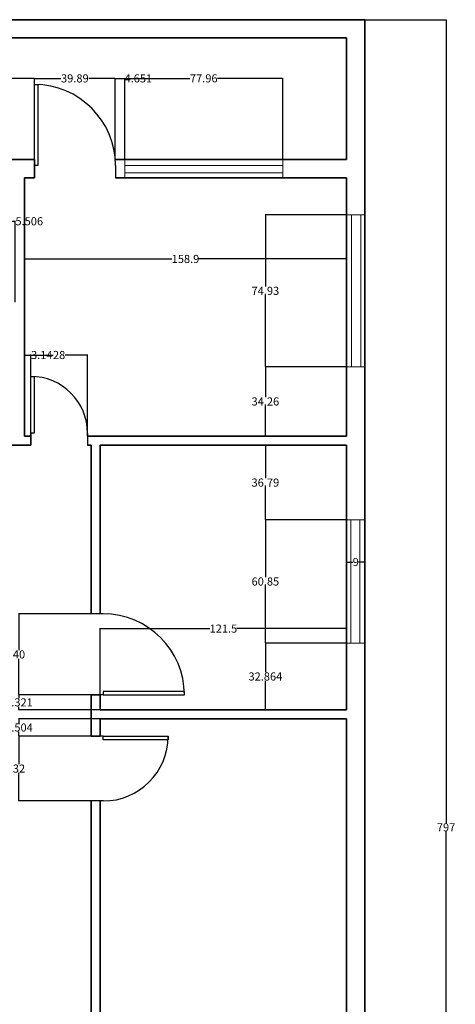
# Model space of a CAD drawing. Units: inches. Extents: x 1353 to 1853, y 16593 to 17433.
# Tile 4 of 4: x 1639 to 1853, y 16947 to 17433. Entities that reach past the tile are written whole.
import ezdxf

# ---------------------------------------------------------------- set-up
doc = ezdxf.new("R2010")
doc.units = ezdxf.units.IN
doc.header["$MEASUREMENT"] = 0
for name, color, linetype, lineweight in [('A-ANNO-DIMS', 2, 'Continuous', 18), ('A-DOOR', 3, 'Continuous', 25), ('A-GLAZ', 4, 'Continuous', 18), ('A-WALL', 7, 'Continuous', 35)]:
    doc.layers.add(name, color=color, linetype=linetype, lineweight=lineweight)
doc.styles.get("Standard").update_dxf_attribs({"font": 'arial.ttf'})
doc.dimstyles.get("Standard").update_dxf_attribs({"dimtxt": 4, "dimasz": 0.18, "dimexe": 0.18, "dimexo": 0.0625, "dimgap": 0.09, "dimtad": 0, "dimtih": 1, "dimtoh": 1, "dimdec": 0, "dimzin": 0, "dimdsep": 46, "dimlunit": 3, "dimtxsty": 'Standard', "dimcen": 0.09, "dimadec": 0, "dimazin": 0, "dimtfac": 1, "dimtdec": 0, "dimtofl": 0, "dimtmove": 0, "dimatfit": 3, "dimfxl": 1, "dimtolj": 1, "dimtzin": 0, "dimarcsym": 0})

# ---------------------------------------------------------------- blocks, each defined once
blk = doc.blocks.new('*U2')
for p, q in [((0, 0), (0, -6)), ((40, 0), (40, -6))]:
    blk.add_line(p, q)
blk.add_lwpolyline([(0, 0), (0, 40), (1.75, 40), (1.75, 0)], close=True)
blk.add_arc((0, 0), 40, 0, 90)
blk = doc.blocks.new('*U6')
for p, q in [((0, 0), (0, -6)), ((28, 0), (28, -6))]:
    blk.add_line(p, q)
blk.add_lwpolyline([(0, 0), (0, 28), (1.75, 28), (1.75, 0)], close=True)
blk.add_arc((0, 0), 28, 0, 90)
blk = doc.blocks.new('*U5')
for p, q in [((0, 0), (0, 6)), ((40, 0), (40, 6))]:
    blk.add_line(p, q)
blk.add_lwpolyline([(0, 0), (0, -40), (1.75, -40), (1.75, 0)], close=True)
blk.add_arc((0, 0), 40, 270, 0)
blk = doc.blocks.new('*U4')
for p, q in [((0, 0), (0, -6)), ((32, 0), (32, -6))]:
    blk.add_line(p, q)
blk.add_lwpolyline([(0, 0), (0, 32), (1.75, 32), (1.75, 0)], close=True)
blk.add_arc((0, 0), 32, 0, 90)
blk = doc.blocks.new('*D14')
at = {"layer": 'A-ANNO-DIMS', "color": 0, "lineweight": -2, "transparency": 16777216}
for p, q in [((1808.95, 17432.78), (1849.11, 17432.78)), ((1848.93, 17432.6), (1848.93, 17036.41)), ((1848.93, 16635.96), (1848.93, 17032.15)), ((1808.95, 16635.78), (1849.11, 16635.78))]:
    blk.add_line(p, q, dxfattribs=at)
at = {"layer": 'A-ANNO-DIMS', "color": 0, "transparency": 16777216}
for points in [[(1848.9, 17432.6), (1848.96, 17432.6), (1848.93, 17432.78)], [(1848.9, 16635.96), (1848.96, 16635.96), (1848.93, 16635.78)]]:
    blk.add_solid(points, dxfattribs=at)
at = {"layer": 'Defpoints', "color": 0, "transparency": 16777216}
for p in [(1808.88, 17432.78), (1848.93, 17432.78), (1808.88, 16635.78)]:
    blk.add_point(p, dxfattribs=at)
at = {"layer": 'A-ANNO-DIMS', "color": 0, "transparency": 16777216, "insert": (1848.93, 17034.28), "char_height": 4, "attachment_point": 5}
blk.add_mtext('\\A1;797', dxfattribs=at)
blk = doc.blocks.new('*D25')
at = {"layer": 'A-ANNO-DIMS', "color": 0, "lineweight": -2, "transparency": 16777216}
for p, q in [((1640.98, 17354.72), (1640.98, 17314.55)), ((1799.88, 17354.72), (1799.88, 17314.55)), ((1641.16, 17314.73), (1713.78, 17314.73)), ((1799.7, 17314.73), (1727.09, 17314.73))]:
    blk.add_line(p, q, dxfattribs=at)
at = {"layer": 'A-ANNO-DIMS', "color": 0, "transparency": 16777216}
for points in [[(1641.16, 17314.76), (1641.16, 17314.7), (1640.98, 17314.73)], [(1799.7, 17314.76), (1799.7, 17314.7), (1799.88, 17314.73)]]:
    blk.add_solid(points, dxfattribs=at)
at = {"layer": 'Defpoints', "color": 0, "transparency": 16777216}
for p in [(1640.98, 17354.78), (1799.88, 17354.78), (1640.98, 17314.73)]:
    blk.add_point(p, dxfattribs=at)
at = {"layer": 'A-ANNO-DIMS', "color": 0, "transparency": 16777216, "insert": (1720.43, 17314.73), "char_height": 4, "attachment_point": 5}
blk.add_mtext('\\A1;158.9', dxfattribs=at)
blk = doc.blocks.new('*D28')
at = {"layer": 'A-ANNO-DIMS', "color": 0, "lineweight": -2, "transparency": 16777216}
for p, q in [((1678.38, 17092.34), (1678.38, 17132.51)), ((1678.56, 17132.33), (1732.47, 17132.33)), ((1799.7, 17132.33), (1745.8, 17132.33)), ((1799.88, 17092.34), (1799.88, 17132.51))]:
    blk.add_line(p, q, dxfattribs=at)
at = {"layer": 'A-ANNO-DIMS', "color": 0, "transparency": 16777216}
for points in [[(1678.56, 17132.36), (1678.56, 17132.3), (1678.38, 17132.33)], [(1799.7, 17132.36), (1799.7, 17132.3), (1799.88, 17132.33)]]:
    blk.add_solid(points, dxfattribs=at)
at = {"layer": 'Defpoints', "color": 0, "transparency": 16777216}
for p in [(1799.88, 17132.33), (1678.38, 17092.28), (1799.88, 17092.28)]:
    blk.add_point(p, dxfattribs=at)
at = {"layer": 'A-ANNO-DIMS', "color": 0, "transparency": 16777216, "insert": (1739.13, 17132.33), "char_height": 4, "attachment_point": 5}
blk.add_mtext('\\A1;121.5', dxfattribs=at)
blk = doc.blocks.new('*D35')
at = {"layer": 'A-ANNO-DIMS', "color": 0, "lineweight": -2, "transparency": 16777216}
for p, q in [((1645.93, 17363.84), (1645.93, 17404.01)), ((1646.11, 17403.83), (1659.03, 17403.83)), ((1685.64, 17403.83), (1672.72, 17403.83)), ((1685.82, 17363.84), (1685.82, 17404.01))]:
    blk.add_line(p, q, dxfattribs=at)
at = {"layer": 'A-ANNO-DIMS', "color": 0, "transparency": 16777216}
for points in [[(1646.11, 17403.86), (1646.11, 17403.8), (1645.93, 17403.83)], [(1685.64, 17403.86), (1685.64, 17403.8), (1685.82, 17403.83)]]:
    blk.add_solid(points, dxfattribs=at)
at = {"layer": 'Defpoints', "color": 0, "transparency": 16777216}
for p in [(1685.82, 17403.83), (1645.93, 17363.78), (1685.82, 17363.78)]:
    blk.add_point(p, dxfattribs=at)
at = {"layer": 'A-ANNO-DIMS', "color": 0, "transparency": 16777216, "insert": (1665.87, 17403.83), "char_height": 4, "attachment_point": 5}
blk.add_mtext('\\A1;39.89', dxfattribs=at)
blk = doc.blocks.new('*D36')
at = {"layer": 'A-ANNO-DIMS', "color": 0, "lineweight": -2, "transparency": 16777216}
for p, q in [((1690.47, 17363.84), (1690.47, 17404.01)), ((1690.65, 17403.83), (1722.63, 17403.83)), ((1768.25, 17403.83), (1736.27, 17403.83)), ((1768.43, 17363.84), (1768.43, 17404.01))]:
    blk.add_line(p, q, dxfattribs=at)
at = {"layer": 'A-ANNO-DIMS', "color": 0, "transparency": 16777216}
for points in [[(1690.65, 17403.86), (1690.65, 17403.8), (1690.47, 17403.83)], [(1768.25, 17403.86), (1768.25, 17403.8), (1768.43, 17403.83)]]:
    blk.add_solid(points, dxfattribs=at)
at = {"layer": 'Defpoints', "color": 0, "transparency": 16777216}
for p in [(1768.43, 17403.83), (1690.47, 17363.78), (1768.43, 17363.78)]:
    blk.add_point(p, dxfattribs=at)
at = {"layer": 'A-ANNO-DIMS', "color": 0, "transparency": 16777216, "insert": (1729.45, 17403.83), "char_height": 4, "attachment_point": 5}
blk.add_mtext('\\A1;77.96', dxfattribs=at)
blk = doc.blocks.new('*D40')
at = {"layer": 'A-ANNO-DIMS', "color": 0, "lineweight": -2, "transparency": 16777216}
for p, q in [((1604.95, 17363.84), (1604.95, 17404.01)), ((1605.13, 17403.83), (1618.52, 17403.83)), ((1645.75, 17403.83), (1632.36, 17403.83)), ((1645.93, 17363.84), (1645.93, 17404.01))]:
    blk.add_line(p, q, dxfattribs=at)
at = {"layer": 'A-ANNO-DIMS', "color": 0, "transparency": 16777216}
for points in [[(1605.13, 17403.86), (1605.13, 17403.8), (1604.95, 17403.83)], [(1645.75, 17403.86), (1645.75, 17403.8), (1645.93, 17403.83)]]:
    blk.add_solid(points, dxfattribs=at)
at = {"layer": 'Defpoints', "color": 0, "transparency": 16777216}
for p in [(1645.93, 17403.83), (1604.95, 17363.78), (1645.93, 17363.78)]:
    blk.add_point(p, dxfattribs=at)
at = {"layer": 'A-ANNO-DIMS', "color": 0, "transparency": 16777216, "insert": (1625.44, 17403.83), "char_height": 4, "attachment_point": 5}
blk.add_mtext('\\A1;40.98', dxfattribs=at)
blk = doc.blocks.new('*D41')
at = {"layer": 'A-ANNO-DIMS', "color": 0, "lineweight": -2, "transparency": 16777216}
for p, q in [((1685.82, 17363.84), (1685.82, 17404.01)), ((1686, 17403.83), (1690.29, 17403.83)), ((1690.47, 17363.84), (1690.47, 17404.01)), ((1690.47, 17403.83), (1690.65, 17403.83))]:
    blk.add_line(p, q, dxfattribs=at)
at = {"layer": 'A-ANNO-DIMS', "color": 0, "transparency": 16777216}
for points in [[(1686, 17403.86), (1686, 17403.8), (1685.82, 17403.83)], [(1690.29, 17403.86), (1690.29, 17403.8), (1690.47, 17403.83)]]:
    blk.add_solid(points, dxfattribs=at)
at = {"layer": 'Defpoints', "color": 0, "transparency": 16777216}
for p in [(1690.47, 17403.83), (1685.82, 17363.78), (1690.47, 17363.78)]:
    blk.add_point(p, dxfattribs=at)
at = {"layer": 'A-ANNO-DIMS', "color": 0, "transparency": 16777216, "insert": (1697.18, 17403.83), "char_height": 4, "attachment_point": 5}
blk.add_mtext('\\A1;4.651', dxfattribs=at)
blk = doc.blocks.new('*D42')
at = {"layer": 'A-ANNO-DIMS', "color": 0, "lineweight": -2, "transparency": 16777216}
for p, q in [((1799.82, 17336.46), (1759.65, 17336.46)), ((1759.83, 17336.28), (1759.83, 17301.13)), ((1759.83, 17261.72), (1759.83, 17296.87)), ((1799.82, 17261.54), (1759.65, 17261.54))]:
    blk.add_line(p, q, dxfattribs=at)
at = {"layer": 'A-ANNO-DIMS', "color": 0, "transparency": 16777216}
for points in [[(1759.8, 17336.28), (1759.86, 17336.28), (1759.83, 17336.46)], [(1759.8, 17261.72), (1759.86, 17261.72), (1759.83, 17261.54)]]:
    blk.add_solid(points, dxfattribs=at)
at = {"layer": 'Defpoints', "color": 0, "transparency": 16777216}
for p in [(1759.83, 17336.46), (1799.88, 17336.46), (1799.88, 17261.54)]:
    blk.add_point(p, dxfattribs=at)
at = {"layer": 'A-ANNO-DIMS', "color": 0, "transparency": 16777216, "insert": (1759.83, 17299), "char_height": 4, "attachment_point": 5}
blk.add_mtext('\\A1;74.93', dxfattribs=at)
blk = doc.blocks.new('*D43')
at = {"layer": 'A-ANNO-DIMS', "color": 0, "lineweight": -2, "transparency": 16777216}
for p, q in [((1799.82, 17261.54), (1759.65, 17261.54)), ((1759.83, 17261.36), (1759.83, 17246.54)), ((1759.83, 17227.46), (1759.83, 17242.28)), ((1799.82, 17227.28), (1759.65, 17227.28))]:
    blk.add_line(p, q, dxfattribs=at)
at = {"layer": 'A-ANNO-DIMS', "color": 0, "transparency": 16777216}
for points in [[(1759.8, 17261.36), (1759.86, 17261.36), (1759.83, 17261.54)], [(1759.8, 17227.46), (1759.86, 17227.46), (1759.83, 17227.28)]]:
    blk.add_solid(points, dxfattribs=at)
at = {"layer": 'Defpoints', "color": 0, "transparency": 16777216}
for p in [(1759.83, 17261.54), (1799.88, 17261.54), (1799.88, 17227.28)]:
    blk.add_point(p, dxfattribs=at)
at = {"layer": 'A-ANNO-DIMS', "color": 0, "transparency": 16777216, "insert": (1759.83, 17244.41), "char_height": 4, "attachment_point": 5}
blk.add_mtext('\\A1;34.26', dxfattribs=at)
blk = doc.blocks.new('*D44')
at = {"layer": 'A-ANNO-DIMS', "color": 0, "lineweight": -2, "transparency": 16777216}
for p, q in [((1799.82, 17185.99), (1759.65, 17185.99)), ((1759.83, 17185.81), (1759.83, 17157.7)), ((1759.83, 17125.32), (1759.83, 17153.44)), ((1799.82, 17125.14), (1759.65, 17125.14))]:
    blk.add_line(p, q, dxfattribs=at)
at = {"layer": 'A-ANNO-DIMS', "color": 0, "transparency": 16777216}
for points in [[(1759.8, 17185.81), (1759.86, 17185.81), (1759.83, 17185.99)], [(1759.8, 17125.32), (1759.86, 17125.32), (1759.83, 17125.14)]]:
    blk.add_solid(points, dxfattribs=at)
at = {"layer": 'Defpoints', "color": 0, "transparency": 16777216}
for p in [(1759.83, 17185.99), (1799.88, 17185.99), (1799.88, 17125.14)]:
    blk.add_point(p, dxfattribs=at)
at = {"layer": 'A-ANNO-DIMS', "color": 0, "transparency": 16777216, "insert": (1759.83, 17155.57), "char_height": 4, "attachment_point": 5}
blk.add_mtext('\\A1;60.85', dxfattribs=at)
blk = doc.blocks.new('*D45')
at = {"layer": 'A-ANNO-DIMS', "color": 0, "lineweight": -2, "transparency": 16777216}
for p, q in [((1799.82, 17125.14), (1759.65, 17125.14)), ((1759.83, 17124.96), (1759.83, 17110.85)), ((1759.83, 17092.46), (1759.83, 17106.58)), ((1799.82, 17092.28), (1759.65, 17092.28))]:
    blk.add_line(p, q, dxfattribs=at)
at = {"layer": 'A-ANNO-DIMS', "color": 0, "transparency": 16777216}
for points in [[(1759.8, 17124.96), (1759.86, 17124.96), (1759.83, 17125.14)], [(1759.8, 17092.46), (1759.86, 17092.46), (1759.83, 17092.28)]]:
    blk.add_solid(points, dxfattribs=at)
at = {"layer": 'Defpoints', "color": 0, "transparency": 16777216}
for p in [(1759.83, 17125.14), (1799.88, 17125.14), (1799.88, 17092.28)]:
    blk.add_point(p, dxfattribs=at)
at = {"layer": 'A-ANNO-DIMS', "color": 0, "transparency": 16777216, "insert": (1759.83, 17108.71), "char_height": 4, "attachment_point": 5}
blk.add_mtext('\\A1;32.864', dxfattribs=at)
blk = doc.blocks.new('*D46')
at = {"layer": 'A-ANNO-DIMS', "color": 0, "lineweight": -2, "transparency": 16777216}
for p, q in [((1799.82, 17222.78), (1759.65, 17222.78)), ((1759.83, 17222.6), (1759.83, 17206.52)), ((1759.83, 17186.17), (1759.83, 17202.25)), ((1799.82, 17185.99), (1759.65, 17185.99))]:
    blk.add_line(p, q, dxfattribs=at)
at = {"layer": 'A-ANNO-DIMS', "color": 0, "transparency": 16777216}
for points in [[(1759.8, 17222.6), (1759.86, 17222.6), (1759.83, 17222.78)], [(1759.8, 17186.17), (1759.86, 17186.17), (1759.83, 17185.99)]]:
    blk.add_solid(points, dxfattribs=at)
at = {"layer": 'Defpoints', "color": 0, "transparency": 16777216}
for p in [(1759.83, 17222.78), (1799.88, 17222.78), (1799.88, 17185.99)]:
    blk.add_point(p, dxfattribs=at)
at = {"layer": 'A-ANNO-DIMS', "color": 0, "transparency": 16777216, "insert": (1759.83, 17204.39), "char_height": 4, "attachment_point": 5}
blk.add_mtext('\\A1;36.79', dxfattribs=at)
blk = doc.blocks.new('*D52')
at = {"layer": 'A-ANNO-DIMS', "color": 0, "lineweight": -2, "transparency": 16777216}
for p, q in [((1630.88, 17293.34), (1630.88, 17333.51)), ((1631.06, 17333.33), (1636.2, 17333.33)), ((1636.38, 17293.34), (1636.38, 17333.51)), ((1636.38, 17333.33), (1636.56, 17333.33))]:
    blk.add_line(p, q, dxfattribs=at)
at = {"layer": 'A-ANNO-DIMS', "color": 0, "transparency": 16777216}
for points in [[(1631.06, 17333.36), (1631.06, 17333.3), (1630.88, 17333.33)], [(1636.2, 17333.36), (1636.2, 17333.3), (1636.38, 17333.33)]]:
    blk.add_solid(points, dxfattribs=at)
at = {"layer": 'Defpoints', "color": 0, "transparency": 16777216}
for p in [(1636.38, 17333.33), (1630.88, 17293.28), (1636.38, 17293.28)]:
    blk.add_point(p, dxfattribs=at)
at = {"layer": 'A-ANNO-DIMS', "color": 0, "transparency": 16777216, "insert": (1643.4, 17333.33), "char_height": 4, "attachment_point": 5}
blk.add_mtext('\\A1;5.506', dxfattribs=at)
blk = doc.blocks.new('*D53')
at = {"layer": 'A-ANNO-DIMS', "color": 0, "lineweight": -2, "transparency": 16777216}
for p, q in [((1644.12, 17227.34), (1644.12, 17267.51)), ((1644.3, 17267.33), (1655.13, 17267.33)), ((1671.94, 17267.33), (1661.12, 17267.33)), ((1672.12, 17227.34), (1672.12, 17267.51))]:
    blk.add_line(p, q, dxfattribs=at)
at = {"layer": 'A-ANNO-DIMS', "color": 0, "transparency": 16777216}
for points in [[(1644.3, 17267.36), (1644.3, 17267.3), (1644.12, 17267.33)], [(1671.94, 17267.36), (1671.94, 17267.3), (1672.12, 17267.33)]]:
    blk.add_solid(points, dxfattribs=at)
at = {"layer": 'Defpoints', "color": 0, "transparency": 16777216}
for p in [(1672.12, 17267.33), (1644.12, 17227.28), (1672.12, 17227.28)]:
    blk.add_point(p, dxfattribs=at)
at = {"layer": 'A-ANNO-DIMS', "color": 0, "transparency": 16777216, "insert": (1658.12, 17267.33), "char_height": 4, "attachment_point": 5}
blk.add_mtext('\\A1;28', dxfattribs=at)
blk = doc.blocks.new('*D54')
at = {"layer": 'A-ANNO-DIMS', "color": 0, "lineweight": -2, "transparency": 16777216}
for p, q in [((1640.98, 17227.34), (1640.98, 17267.51)), ((1641.16, 17267.33), (1643.94, 17267.33)), ((1644.12, 17227.34), (1644.12, 17267.51)), ((1644.12, 17267.33), (1644.3, 17267.33))]:
    blk.add_line(p, q, dxfattribs=at)
at = {"layer": 'A-ANNO-DIMS', "color": 0, "transparency": 16777216}
for points in [[(1641.16, 17267.36), (1641.16, 17267.3), (1640.98, 17267.33)], [(1643.94, 17267.36), (1643.94, 17267.3), (1644.12, 17267.33)]]:
    blk.add_solid(points, dxfattribs=at)
at = {"layer": 'Defpoints', "color": 0, "transparency": 16777216}
for p in [(1644.12, 17267.33), (1640.98, 17227.28), (1644.12, 17227.28)]:
    blk.add_point(p, dxfattribs=at)
at = {"layer": 'A-ANNO-DIMS', "color": 0, "transparency": 16777216, "insert": (1649.58, 17267.33), "char_height": 4, "attachment_point": 5}
blk.add_mtext('\\A1;3.14', dxfattribs=at)
blk = doc.blocks.new('*D61')
at = {"layer": 'A-ANNO-DIMS', "color": 0, "lineweight": -2, "transparency": 16777216}
for p, q in [((1678.32, 17139.6), (1638.15, 17139.6)), ((1638.33, 17139.42), (1638.33, 17121.73)), ((1638.33, 17099.78), (1638.33, 17117.47)), ((1678.32, 17099.6), (1638.15, 17099.6))]:
    blk.add_line(p, q, dxfattribs=at)
at = {"layer": 'A-ANNO-DIMS', "color": 0, "transparency": 16777216}
for points in [[(1638.3, 17139.42), (1638.36, 17139.42), (1638.33, 17139.6)], [(1638.3, 17099.78), (1638.36, 17099.78), (1638.33, 17099.6)]]:
    blk.add_solid(points, dxfattribs=at)
at = {"layer": 'Defpoints', "color": 0, "transparency": 16777216}
for p in [(1638.33, 17139.6), (1678.38, 17139.6), (1678.38, 17099.6)]:
    blk.add_point(p, dxfattribs=at)
at = {"layer": 'A-ANNO-DIMS', "color": 0, "transparency": 16777216, "insert": (1638.33, 17119.6), "char_height": 4, "attachment_point": 5}
blk.add_mtext('\\A1;40', dxfattribs=at)
blk = doc.blocks.new('*D62')
at = {"layer": 'A-ANNO-DIMS', "color": 0, "lineweight": -2, "transparency": 16777216}
for p, q in [((1678.32, 17079.28), (1638.15, 17079.28)), ((1638.33, 17079.1), (1638.33, 17065.41)), ((1638.33, 17047.46), (1638.33, 17061.14)), ((1678.32, 17047.28), (1638.15, 17047.28))]:
    blk.add_line(p, q, dxfattribs=at)
at = {"layer": 'A-ANNO-DIMS', "color": 0, "transparency": 16777216}
for points in [[(1638.3, 17079.1), (1638.36, 17079.1), (1638.33, 17079.28)], [(1638.3, 17047.46), (1638.36, 17047.46), (1638.33, 17047.28)]]:
    blk.add_solid(points, dxfattribs=at)
at = {"layer": 'Defpoints', "color": 0, "transparency": 16777216}
for p in [(1638.33, 17079.28), (1678.38, 17079.28), (1678.38, 17047.28)]:
    blk.add_point(p, dxfattribs=at)
at = {"layer": 'A-ANNO-DIMS', "color": 0, "transparency": 16777216, "insert": (1638.33, 17063.28), "char_height": 4, "attachment_point": 5}
blk.add_mtext('\\A1;32', dxfattribs=at)
blk = doc.blocks.new('*D74')
at = {"layer": 'A-ANNO-DIMS', "color": 0, "lineweight": -2, "transparency": 16777216}
for p, q in [((1678.32, 17087.78), (1638.15, 17087.78)), ((1638.33, 17087.6), (1638.33, 17085.66)), ((1678.32, 17079.28), (1638.15, 17079.28)), ((1638.33, 17079.46), (1638.33, 17081.4))]:
    blk.add_line(p, q, dxfattribs=at)
at = {"layer": 'A-ANNO-DIMS', "color": 0, "transparency": 16777216}
for points in [[(1638.3, 17087.6), (1638.36, 17087.6), (1638.33, 17087.78)], [(1638.3, 17079.46), (1638.36, 17079.46), (1638.33, 17079.28)]]:
    blk.add_solid(points, dxfattribs=at)
at = {"layer": 'Defpoints', "color": 0, "transparency": 16777216}
for p in [(1638.33, 17087.78), (1678.38, 17087.78), (1678.38, 17079.28)]:
    blk.add_point(p, dxfattribs=at)
at = {"layer": 'A-ANNO-DIMS', "color": 0, "transparency": 16777216, "insert": (1638.33, 17083.53), "char_height": 4, "attachment_point": 5}
blk.add_mtext('\\A1;8.504', dxfattribs=at)
blk = doc.blocks.new('*D75')
at = {"layer": 'A-ANNO-DIMS', "color": 0, "lineweight": -2, "transparency": 16777216}
for p, q in [((1678.32, 17099.6), (1638.15, 17099.6)), ((1638.33, 17099.42), (1638.33, 17098.08)), ((1678.32, 17092.28), (1638.15, 17092.28)), ((1638.33, 17092.46), (1638.33, 17093.81))]:
    blk.add_line(p, q, dxfattribs=at)
at = {"layer": 'A-ANNO-DIMS', "color": 0, "transparency": 16777216}
for points in [[(1638.3, 17099.42), (1638.36, 17099.42), (1638.33, 17099.6)], [(1638.3, 17092.46), (1638.36, 17092.46), (1638.33, 17092.28)]]:
    blk.add_solid(points, dxfattribs=at)
at = {"layer": 'Defpoints', "color": 0, "transparency": 16777216}
for p in [(1638.33, 17099.6), (1678.38, 17099.6), (1678.38, 17092.28)]:
    blk.add_point(p, dxfattribs=at)
at = {"layer": 'A-ANNO-DIMS', "color": 0, "transparency": 16777216, "insert": (1638.33, 17095.94), "char_height": 4, "attachment_point": 5}
blk.add_mtext('\\A1;7.321', dxfattribs=at)
blk = doc.blocks.new('*D78')
at = {"layer": 'A-ANNO-DIMS', "color": 0, "lineweight": -2, "transparency": 16777216}
for p, q in [((1799.88, 17125.21), (1799.88, 17165.37)), ((1800.06, 17165.19), (1802.98, 17165.19)), ((1808.7, 17165.19), (1805.79, 17165.19)), ((1808.88, 17125.21), (1808.88, 17165.37))]:
    blk.add_line(p, q, dxfattribs=at)
at = {"layer": 'A-ANNO-DIMS', "color": 0, "transparency": 16777216}
for points in [[(1800.06, 17165.22), (1800.06, 17165.16), (1799.88, 17165.19)], [(1808.7, 17165.22), (1808.7, 17165.16), (1808.88, 17165.19)]]:
    blk.add_solid(points, dxfattribs=at)
at = {"layer": 'Defpoints', "color": 0, "transparency": 16777216}
for p in [(1808.88, 17165.19), (1799.88, 17125.14), (1808.88, 17125.14)]:
    blk.add_point(p, dxfattribs=at)
at = {"layer": 'A-ANNO-DIMS', "color": 0, "transparency": 16777216, "insert": (1804.38, 17165.19), "char_height": 4, "attachment_point": 5}
blk.add_mtext('\\A1;9', dxfattribs=at)

msp = doc.modelspace()

# ---------------------------------------------------------------- linework, layer by layer
at = {"layer": 'A-GLAZ'}
for p, q in [((1690.4681, 17363.7809), (1690.4681, 17354.7809)), ((1768.4275, 17363.7809), (1690.4681, 17363.7809)), ((1690.4681, 17363.7809), (1690.4681, 17360.9071)), ((1768.4275, 17354.7809), (1768.4275, 17363.7809)), ((1690.4681, 17360.9071), (1768.4275, 17360.9071)), ((1768.4275, 17360.9071), (1768.4275, 17357.2518)), ((1768.4275, 17357.2518), (1690.4681, 17357.2518)), ((1690.4681, 17354.7809), (1768.4275, 17354.7809)), ((1799.8844, 17336.4635), (1808.8844, 17336.4635)), ((1799.8844, 17261.5382), (1799.8844, 17336.4635)), ((1799.8844, 17336.4635), (1802.3172, 17336.4635)), ((1802.3172, 17336.4635), (1802.3172, 17261.5382)), ((1806.8587, 17261.5382), (1806.8587, 17336.4635)), ((1808.8844, 17336.4635), (1808.8844, 17261.5382)), ((1808.8844, 17261.5382), (1799.8844, 17261.5382)), ((1802.3172, 17261.5382), (1806.8587, 17261.5382)), ((1799.8844, 17185.9944), (1808.8844, 17185.9944)), ((1799.8844, 17125.1449), (1799.8844, 17185.9944)), ((1799.8844, 17185.9944), (1801.8923, 17185.9944)), ((1801.8923, 17185.9944), (1801.8923, 17125.1449)), ((1806.3721, 17125.1449), (1806.3721, 17185.9944)), ((1808.8844, 17185.9944), (1808.8844, 17125.1449)), ((1808.8844, 17125.1449), (1799.8844, 17125.1449)), ((1801.8923, 17125.1449), (1806.3721, 17125.1449))]:
    msp.add_line(p, q, dxfattribs=at)
at = {"layer": 'A-WALL'}
for p, q in [((1388.8844, 17432.7809), (1808.8844, 17432.7809)), ((1808.8844, 17432.7809), (1808.8844, 16635.7809)), ((1397.8844, 17423.7809), (1799.8844, 17423.7809)), ((1799.8844, 17423.7809), (1799.8844, 17363.7809)), ((1459.183, 17363.7809), (1645.9302, 17363.7809)), ((1645.9302, 17354.7809), (1645.9302, 17363.7809)), ((1688.5176, 17363.7809), (1685.8175, 17363.7809)), ((1688.5176, 17363.7809), (1799.8844, 17363.7809)), ((1640.9844, 17227.2809), (1640.9844, 17354.7809)), ((1640.9844, 17354.7809), (1645.9302, 17354.7809)), ((1690.4681, 17354.7809), (1685.9302, 17354.7809)), ((1688.5176, 17354.7809), (1799.8844, 17354.7809)), ((1799.8844, 17354.7809), (1799.8844, 17227.2809)), ((1640.9844, 17227.2809), (1644.1249, 17227.2809)), ((1644.1249, 17222.7809), (1644.1249, 17227.2809)), ((1672.1249, 17227.2809), (1799.8844, 17227.2809)), ((1528.3844, 17222.7809), (1640.9844, 17222.7809)), ((1640.9844, 17222.7809), (1644.1249, 17222.7809)), ((1672.1249, 17222.7809), (1673.8844, 17222.7809)), ((1673.8844, 17222.7809), (1673.8844, 17139.6023)), ((1678.3844, 17222.7809), (1678.3844, 17139.6023)), ((1678.3844, 17222.7809), (1799.8844, 17222.7809)), ((1799.8844, 17222.7809), (1799.8844, 17092.2809)), ((1678.3844, 17099.6023), (1673.8844, 17099.6023)), ((1673.8844, 17087.7809), (1673.8844, 17099.6023)), ((1673.8844, 17099.6023), (1678.3844, 17099.6023)), ((1678.3844, 17099.6023), (1678.3844, 17092.2809)), ((1678.3844, 17092.2809), (1799.8844, 17092.2809)), ((1673.8844, 17087.7809), (1673.8844, 17079.277)), ((1678.3844, 17087.7809), (1799.8844, 17087.7809)), ((1678.3844, 17087.7809), (1678.3844, 17079.277)), ((1799.8844, 17087.7809), (1799.8844, 16644.7809)), ((1678.3844, 17079.277), (1673.8844, 17079.277)), ((1673.8844, 16893.7809), (1673.8844, 17047.277)), ((1678.3844, 16759.1207), (1678.3844, 17047.277))]:
    msp.add_line(p, q, dxfattribs=at)

# ---------------------------------------------------------------- block references
at = {"layer": 'A-DOOR'}
for name, p in [('*U2', (1645.9302, 17360.7809)), ('*U6', (1644.1249, 17228.7809))]:
    msp.add_blockref(name, p, dxfattribs=at)
for name, p, rotation in [('*U5', (1679.8844, 17099.6023), 90), ('*U4', (1679.8844, 17079.277), 270.0000000000025)]:
    msp.add_blockref(name, p, dxfattribs=dict(at, rotation=rotation))

# ---------------------------------------------------------------- dimensions: what is measured, and where the dimension line sits
at = {"layer": 'A-ANNO-DIMS'}
for base, p1, p2, angle, override, picture, middle in [((1848.9344, 17432.7809), (1808.8844, 16635.7809), (1808.8844, 17432.7809), 90, {"dimdec": 0, "dimlfac": 1, "dimrnd": 0, "dimzin": 0, "dimdsep": 46, "dimlunit": 2}, '*D14', (1848.9344, 17034.2809)), ((1640.9844, 17314.7309), (1799.8844, 17354.7809), (1640.9844, 17354.7809), 180, {"dimdec": 1, "dimlfac": 1, "dimrnd": 0, "dimzin": 0, "dimdsep": 46, "dimlunit": 2}, '*D25', (1720.4344, 17314.7309)), ((1759.8344, 17336.4635), (1799.8844, 17261.5382), (1799.8844, 17336.4635), 90, {"dimdec": 2, "dimlfac": 1, "dimrnd": 0, "dimzin": 0, "dimdsep": 46, "dimlunit": 2}, '*D42', (1759.8344, 17299.0008)), ((1759.8344, 17261.5382), (1799.8844, 17227.2809), (1799.8844, 17261.5382), 90, {"dimdec": 2, "dimlfac": 1, "dimrnd": 0, "dimzin": 0, "dimdsep": 46, "dimlunit": 2}, '*D43', (1759.8344, 17244.4096)), ((1759.8344, 17222.7809), (1799.8844, 17185.9944), (1799.8844, 17222.7809), 90, {"dimdec": 2, "dimlfac": 1, "dimrnd": 0, "dimzin": 0, "dimdsep": 46, "dimlunit": 2}, '*D46', (1759.8344, 17204.3877)), ((1759.8344, 17185.9944), (1799.8844, 17125.1449), (1799.8844, 17185.9944), 90, {"dimdec": 2, "dimlfac": 1, "dimrnd": 0, "dimzin": 0, "dimdsep": 46, "dimlunit": 2}, '*D44', (1759.8344, 17155.5696)), ((1638.3344, 17139.6023), (1678.3844, 17099.6023), (1678.3844, 17139.6023), 90, {"dimdec": 0, "dimlfac": 1, "dimrnd": 0, "dimzin": 0, "dimdsep": 46, "dimlunit": 2}, '*D61', (1638.3344, 17119.6023)), ((1759.8344, 17125.1449), (1799.8844, 17092.2809), (1799.8844, 17125.1449), 90, {"dimdec": 3, "dimlfac": 1, "dimrnd": 0, "dimzin": 0, "dimdsep": 46, "dimlunit": 2}, '*D45', (1759.8344, 17108.7129)), ((1638.3344, 17099.6023), (1678.3844, 17092.2809), (1678.3844, 17099.6023), 90, {"dimdec": 3, "dimlfac": 1, "dimrnd": 0, "dimzin": 0, "dimdsep": 46, "dimlunit": 2}, '*D75', (1638.3344, 17095.9416)), ((1638.3344, 17087.7809), (1678.3844, 17079.277), (1678.3844, 17087.7809), 90, {"dimdec": 3, "dimlfac": 1, "dimrnd": 0, "dimzin": 0, "dimdsep": 46, "dimlunit": 2}, '*D74', (1638.3344, 17083.529)), ((1638.3344, 17079.277), (1678.3844, 17047.277), (1678.3844, 17079.277), 90, {"dimdec": 0, "dimlfac": 1, "dimrnd": 0, "dimzin": 0, "dimdsep": 46, "dimlunit": 2}, '*D62', (1638.3344, 17063.277))]:
    dim = msp.add_linear_dim(base=base, p1=p1, p2=p2, angle=angle, dimstyle='Standard', override=override, dxfattribs=at)
    dim.commit()
    dim.dimension.update_dxf_attribs({"geometry": picture, "text_midpoint": middle})
for base, p1, p2, override, picture, middle in [((1645.9302, 17403.8309), (1604.9522, 17363.7809), (1645.9302, 17363.7809), {"dimdec": 2, "dimlfac": 1, "dimrnd": 0, "dimzin": 0, "dimdsep": 46, "dimlunit": 2}, '*D40', (1625.4412, 17403.8309)), ((1685.8175, 17403.8309), (1645.9302, 17363.7809), (1685.8175, 17363.7809), {"dimdec": 2, "dimlfac": 1, "dimrnd": 0, "dimzin": 0, "dimdsep": 46, "dimlunit": 2}, '*D35', (1665.8739, 17403.8309)), ((1690.4681, 17403.8309), (1685.8175, 17363.7809), (1690.4681, 17363.7809), {"dimdec": 3, "dimlfac": 1, "dimrnd": 0, "dimzin": 0, "dimdsep": 46, "dimlunit": 2}, '*D41', (1697.1815, 17403.8309)), ((1768.4275, 17403.8309), (1690.4681, 17363.7809), (1768.4275, 17363.7809), {"dimdec": 2, "dimlfac": 1, "dimrnd": 0, "dimzin": 0, "dimdsep": 46, "dimlunit": 2}, '*D36', (1729.4478, 17403.8309)), ((1636.3844, 17333.3309), (1630.8782, 17293.2809), (1636.3844, 17293.2809), {"dimdec": 3, "dimlfac": 1, "dimrnd": 0, "dimzin": 0, "dimdsep": 46, "dimlunit": 2}, '*D52', (1643.402, 17333.3309)), ((1644.1249, 17267.3309), (1640.9844, 17227.2809), (1644.1249, 17227.2809), {"dimdec": 2, "dimlfac": 1, "dimrnd": 0, "dimzin": 0, "dimdsep": 46, "dimlunit": 2}, '*D54', (1649.5804, 17267.3309)), ((1672.1249, 17267.3309), (1644.1249, 17227.2809), (1672.1249, 17227.2809), {"dimdec": 0, "dimlfac": 1, "dimrnd": 0, "dimzin": 0, "dimdsep": 46, "dimlunit": 2}, '*D53', (1658.1249, 17267.3309)), ((1808.8844, 17165.1949), (1799.8844, 17125.1449), (1808.8844, 17125.1449), {"dimdec": 0, "dimlfac": 1, "dimrnd": 0, "dimzin": 0, "dimdsep": 46, "dimlunit": 2}, '*D78', (1804.3844, 17165.1949)), ((1799.8844, 17132.3309), (1678.3844, 17092.2809), (1799.8844, 17092.2809), {"dimdec": 1, "dimlfac": 1, "dimrnd": 0, "dimzin": 0, "dimdsep": 46, "dimlunit": 2}, '*D28', (1739.1344, 17132.3309))]:
    dim = msp.add_linear_dim(base=base, p1=p1, p2=p2, dimstyle='Standard', override=override, dxfattribs=at)
    dim.commit()
    dim.dimension.update_dxf_attribs({"geometry": picture, "text_midpoint": middle})

doc.saveas('drawing.dxf')
